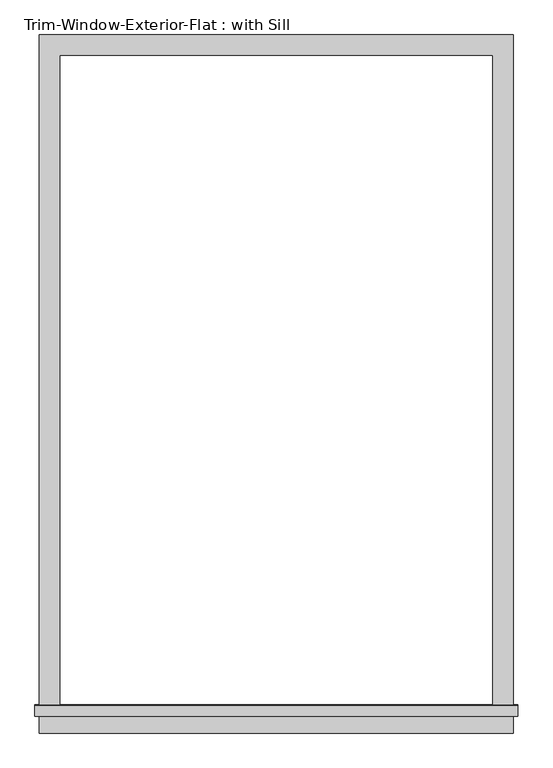
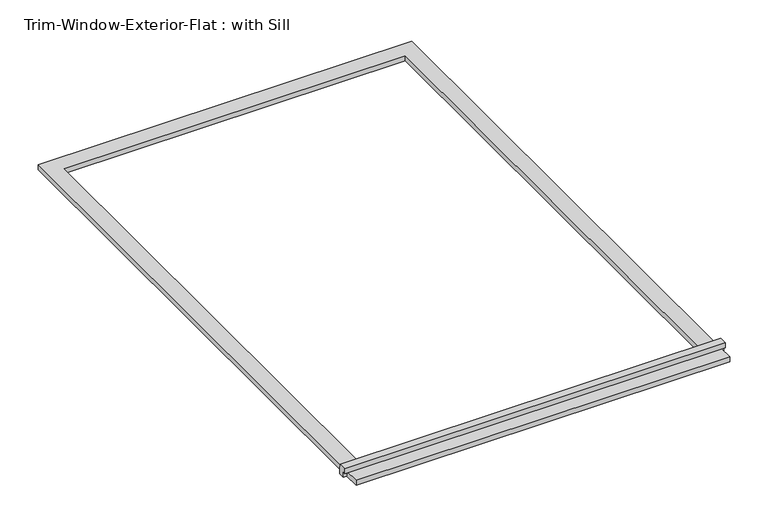
"""IFC4 building model written with IfcOpenShell, lengths in millimetres: proxy geometry, Trim-Window-Exterior-Flat : with Sill."""

from ifc_helpers import new_model, si_unit, frame, origin, origin_with_axes, place, context, project, spatial, polyline, outline, extrude, source, transform, mapped, element, save


def trim_window_exterior_flat_with_sill_b7e4d11c(model_context):
    return source(origin(), model_context, "Body", "SweptSolid", [
        extrude(outline(polyline([(666.75, -1850.9823709), (666.75, -1908.1323709), (-666.75, -1908.1323709), (-666.75, -1850.9823709), (666.75, -1850.9823709)])), origin_with_axes(), (0.0, 0.0, 1.0), 19.05),
        extrude(outline(polyline([(-1860.55, 38.1), (-1831.2580645, 38.1), (-1828.8, 19.05), (-1828.8, 0.0), (-1850.9823709, 0.0), (-1850.9823709, 19.05), (-1860.55, 19.05), (-1860.55, 38.1)])), frame((-679.45, 0.0, 0.0), z_axis=(1.0, 0.0, 0.0), x_axis=(0.0, 1.0, 0.0)), (0.0, 0.0, 1.0), 1358.9),
        extrude(outline(polyline([(-666.75, 57.15), (666.75, 57.15), (666.75, -1828.8), (609.6, -1828.8), (609.6, 0.0), (-609.6, 0.0), (-609.6, -1828.8), (-666.75, -1828.8), (-666.75, 57.15)])), origin_with_axes(), (0.0, 0.0, 1.0), 19.05),
    ])


if __name__ == "__main__":
    model = new_model("IFC4")
    model_context = context("Model", 3, world=origin())
    ifc_project = project(units=[si_unit("LENGTHUNIT", "METRE", prefix="MILLI")], contexts=[model_context])
    site = spatial("IfcSite", under=ifc_project)
    building = spatial("IfcBuilding", under=site)
    placement = place(None, origin())
    trim_window_exterior_flat_with_sill_shape = trim_window_exterior_flat_with_sill_b7e4d11c(model_context)
    element("IfcBuildingElementProxy", 1, Name="Trim-Window-Exterior-Flat : with Sill", ObjectType="Trim-Window-Exterior-Flat : with Sill", at=placement, inside=building, context=model_context, shape_type="MappedRepresentation", body=[
        mapped(trim_window_exterior_flat_with_sill_shape, transform((0.0, 0.0, 0.0), x_axis=(1.0, 0.0, 0.0), y_axis=(0.0, 1.0, 0.0), z_axis=(0.0, 0.0, 1.0))),
    ])
    save(model, "model.ifc")

# Revit data of these elements
# Type "Trim-Window-Exterior-Flat : with Sill"
#   Trim Width = 0' - 2 1/4"
#   Trim Thickness_Picture Frame = 0' - 1 1/4"
#   Trim Thickness_with Sill = 0' - 0 3/4"
#   Sill Thickness = 0' - 1 1/4"
#   Opening Width [instance default] = 2' - 0"
#   Opening Height [instance default] = 3' - 0"
#   Default Elevation = 4' - 0"
#   Sill = yes
#   Picture Frame = no
#   Trim Material [instance default] = none
# Element 1 (IfcBuildingElementProxy, "Trim-Window-Exterior-Flat : with Sill")
#   Opening Width = 4' - 0"
#   Opening Height = 6' - 0"
#   Trim Material = Clad - White
#   Materials on its faces: "Clad - White"
# Materials
#   "Clad - White": class "Wood", colour RGB 242 242 238, transparency 0, Cost = 0
